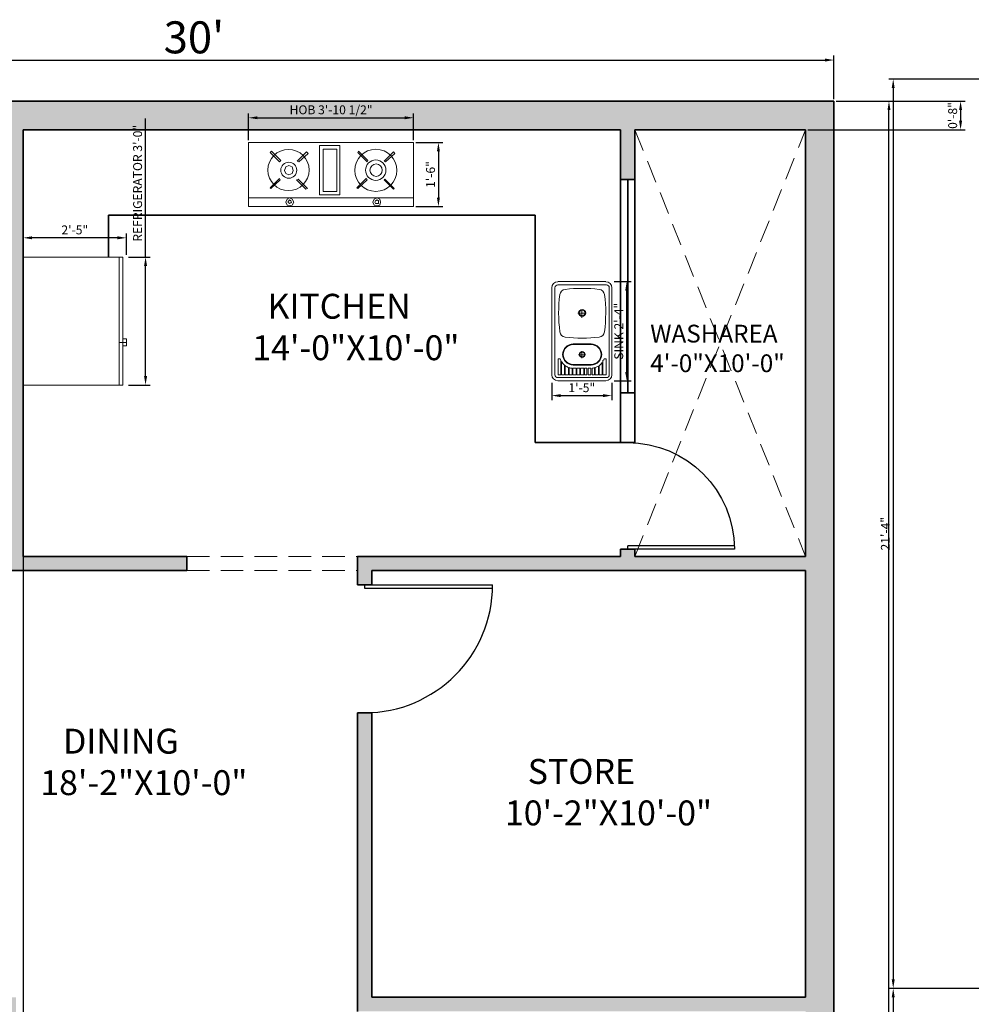
# Model space of a CAD drawing. Units: inches. Extents: x 1566 to 2546, y 1087 to 2705.
# Tile 11 of 27: x 1773 to 2040, y 1524 to 1801. Entities that reach past the tile are written whole.
import ezdxf

# ---------------------------------------------------------------- set-up
doc = ezdxf.new("R2010")
doc.units = ezdxf.units.IN
doc.linetypes.add('DASHED', pattern=[19.05, 12.7, -6.35])
for name, color, linetype, lineweight in [('A-ANNO-DIMS', 2, 'Continuous', 18), ('A-AREA-IDEN', 7, 'Continuous', 18), ('A-DOOR', 4, 'Continuous', 25), ('A-FLOR-FIXT', 9, 'Continuous', 18), ('A-FLOR-OVHD', 8, 'DASHED', 18), ('A-WALL', 7, 'Continuous', 35), ('A-WALL-PATT', 8, 'Continuous', 13)]:
    doc.layers.add(name, color=color, linetype=linetype, lineweight=lineweight)
doc.styles.get("Standard").update_dxf_attribs({"font": 'arial.ttf'})
doc.dimstyles.new('ISO-25', dxfattribs={"dimtxt": 2.5, "dimasz": 2.5, "dimexe": 1.25, "dimexo": 0.625, "dimtad": 1, "dimtxsty": 'Standard', "dimcen": 2.5, "dimadec": 0, "dimazin": 0, "dimtfac": 1, "dimtmove": 0, "dimatfit": 3, "dimfxl": 1, "dimarcsym": 0})

# ---------------------------------------------------------------- blocks, each defined once
blk = doc.blocks.new('d1')
for p, q in [((3297.32, 1596.93), (3297.32, 1632.93)), ((3298.32, 1596.93), (3298.32, 1632.93)), ((3297.32, 1596.93), (3298.32, 1596.93))]:
    blk.add_line(p, q)
at = {"ltscale": 0.3}
blk.add_arc((3297.32, 1596.93), 36, 0, 90, dxfattribs=at)
blk = doc.blocks.new('*D7')
at = {"layer": 'A-ANNO-DIMS', "color": 0, "lineweight": -2, "transparency": 16777216}
for p, q in [((2002.15, 1778.2), (2018.24, 1778.2)), ((2016.99, 1156.7), (2016.99, 1775.7)), ((2002.15, 1154.2), (2018.24, 1154.2))]:
    blk.add_line(p, q, dxfattribs=at)
at = {"layer": 'A-ANNO-DIMS', "color": 0, "transparency": 16777216}
for points in [[(2016.58, 1775.7), (2017.41, 1775.7), (2016.99, 1778.2)], [(2016.58, 1156.7), (2017.41, 1156.7), (2016.99, 1154.2)]]:
    blk.add_solid(points, dxfattribs=at)
at = {"layer": 'Defpoints', "color": 0, "transparency": 16777216}
for p in [(2001.53, 1778.2), (2016.99, 1778.2), (2001.53, 1154.2)]:
    blk.add_point(p, dxfattribs=at)
at = {"layer": 'A-ANNO-DIMS', "color": 0, "transparency": 16777216, "insert": (2011.77, 1466.2), "char_height": 9, "attachment_point": 5, "rotation": 90}
blk.add_mtext("52'", dxfattribs=at)
blk = doc.blocks.new('*D9')
at = {"layer": 'A-ANNO-DIMS', "color": 0, "lineweight": -2, "transparency": 16777216}
for p, q in [((1641.53, 1778.82), (1641.53, 1791.04)), ((1644.03, 1789.79), (1999.03, 1789.79)), ((2001.53, 1778.82), (2001.53, 1791.04))]:
    blk.add_line(p, q, dxfattribs=at)
at = {"layer": 'A-ANNO-DIMS', "color": 0, "transparency": 16777216}
for points in [[(1644.03, 1790.2), (1644.03, 1789.37), (1641.53, 1789.79)], [(1999.03, 1790.2), (1999.03, 1789.37), (2001.53, 1789.79)]]:
    blk.add_solid(points, dxfattribs=at)
at = {"layer": 'Defpoints', "color": 0, "transparency": 16777216}
for p in [(2001.53, 1789.79), (1641.53, 1778.2), (2001.53, 1778.2)]:
    blk.add_point(p, dxfattribs=at)
at = {"layer": 'A-ANNO-DIMS', "color": 0, "transparency": 16777216, "insert": (1821.53, 1795.01), "char_height": 9, "attachment_point": 5}
blk.add_mtext("30'", dxfattribs=at)
blk = doc.blocks.new('d2')
for p, q in [((3364.08, 1632.29), (3364.08, 1602.29)), ((3365.08, 1632.29), (3365.08, 1602.29)), ((3364.08, 1602.29), (3365.08, 1602.29))]:
    blk.add_line(p, q)
at = {"ltscale": 0.3}
blk.add_arc((3364.08, 1602.29), 30, 0, 90, dxfattribs=at)
blk = doc.blocks.new('sink 1')
for points in [[(5.86, 24.22), (-5.86, 24.22)], [(-7.34, 1.48), (-7.34, 22.73)], [(-6.56, 1.48), (-6.56, 22.73)], [(6.01, 23.43), (-5.86, 23.43)], [(6.72, 1.48), (6.72, 22.73)], [(7.34, 1.48), (7.34, 22.73)], [(0, 15.39), (0, 17.42)], [(1.09, 16.48), (-0.94, 16.48)], [(-2.09, 8.99), (2.28, 8.99)], [(-2.09, 8.84), (2.28, 8.84)], [(0, 5.55), (0, 7.26)], [(-5.78, 5.39), (-5.78, 5.39)], [(-5.31, 5.39), (-5.31, 5.39)], [(-5.16, 4.92), (-5.16, 4.92)], [(0.78, 6.33), (-0.78, 6.33)], [(5.16, 4.92), (5.16, 4.92)], [(5.94, 5.39), (5.94, 5.39)], [(-5, 1.48), (-5, 4.69)], [(-5, 1.48), (-4.22, 1.48), (-4.22, 3.83)], [(-4.84, 4.45), (-4.84, 4.45)], [(-4.22, 3.83), (-4.22, 3.83)], [(-4.06, 1.48), (-4.06, 3.69)], [(-4.06, 1.48), (-3.28, 1.48), (-3.28, 3.27)], [(-3.91, 3.52), (-3.91, 3.52)], [(-3.28, 3.2), (-3.28, 3.2)], [(-3.12, 3.2), (-3.12, 3.2)], [(-2.34, 3.05), (-2.34, 3.05)], [(-2.19, 3.05), (-2.19, 3.05)], [(-2.09, 3.99), (2.28, 3.99)], [(-2.09, 3.84), (2.28, 3.84)], [(-1.41, 3.05), (-1.41, 3.05)], [(-1.25, 3.05), (-1.25, 3.05)], [(-0.47, 1.48), (-1.25, 1.48), (-1.25, 3.05), (-0.47, 3.05)], [(-0.62, 3.05), (-0.62, 3.05)], [(-0.47, 1.48), (-0.47, 3.05)], [(-0.31, 3.05), (-0.31, 3.05)], [(0.47, 1.48), (-0.31, 1.48), (-0.31, 3.05), (0.47, 3.05)], [(0.31, 3.05), (0.31, 3.05)], [(0.47, 1.48), (0.47, 3.05)], [(0.62, 3.05), (0.62, 3.05)], [(1.25, 3.05), (1.25, 3.05)], [(1.56, 3.05), (1.56, 3.05)], [(2.19, 3.05), (2.19, 3.05)], [(2.5, 3.05), (2.5, 3.05)], [(3.12, 3.2), (3.12, 3.2)], [(3.28, 1.48), (4.06, 1.48), (4.06, 3.57)], [(3.28, 1.48), (3.28, 3.2)], [(3.44, 3.2), (3.44, 3.2)], [(4.06, 3.52), (4.06, 3.52)], [(4.22, 1.48), (4.22, 3.67)], [(4.37, 3.83), (4.37, 3.83)], [(5, 4.45), (5, 4.45)], [(6.01, 0.78), (-5.86, 0.78)], [(5.86, 0), (-5.86, 0)], [(-5.78, 1.48), (-5.78, 1.48)], [(-5.16, 1.48), (-5.16, 1.48)], [(-4.84, 1.48), (-4.84, 1.48)], [(-4.22, 1.48), (-4.22, 1.48)], [(-3.91, 1.48), (-3.91, 1.48)], [(-3.28, 1.48), (-3.28, 1.48)], [(-3.12, 1.48), (-3.12, 1.48)], [(-2.34, 1.48), (-2.34, 1.48)], [(-2.19, 1.48), (-2.19, 1.48)], [(-1.41, 1.48), (-1.41, 1.48)], [(-1.25, 1.48), (-1.25, 1.48)], [(-0.62, 1.48), (-0.62, 1.48)], [(-0.31, 1.48), (-0.31, 1.48)], [(0.31, 1.48), (0.31, 1.48)], [(0.62, 1.48), (0.62, 1.48)], [(1.25, 1.48), (1.25, 1.48)], [(1.56, 1.48), (1.56, 1.48)], [(2.19, 1.48), (2.19, 1.48)], [(2.5, 1.48), (2.5, 1.48)], [(3.12, 1.48), (3.12, 1.48)], [(3.44, 1.48), (3.44, 1.48)], [(4.06, 1.48), (4.06, 1.48)], [(4.37, 1.48), (4.37, 1.48)], [(5, 1.48), (5, 1.48)], [(5.16, 1.48), (5.16, 1.48)], [(5.94, 1.48), (5.94, 1.48)]]:
    blk.add_lwpolyline(points)
for points in [[(-5.16, 4.92), (-5.16, 1.48), (-5.78, 1.48), (-5.78, 5.39), (-5.31, 5.39, -0.068511), (-5.16, 4.92)], [(5.16, 4.92, 0.248301), (5.47, 5.39), (5.94, 5.39), (5.94, 1.48), (5.16, 1.48), (5.16, 4.92)], [(4.06, 3.57, -0.061679), (3.32, 3.22)], [(4.22, 1.48), (5, 1.48), (5, 4.45, -0.083542), (4.22, 3.67, -0.083542)]]:
    blk.add_lwpolyline(points, format="xyb")
for points in [[(-3.12, 3.22), (-3.12, 1.48), (-2.34, 1.48), (-2.34, 3.05, -0.06228)], [(2.5, 3.05), (2.5, 1.48), (3.12, 1.48), (3.12, 3.2, -0.050256)]]:
    blk.add_lwpolyline(points, format="xyb", close=True)
for points in [[(-2.19, 3.05), (-1.41, 3.05), (-1.41, 1.48), (-2.19, 1.48)], [(0.62, 3.05), (1.25, 3.05), (1.25, 1.48), (0.62, 1.48)], [(2.19, 1.48), (2.19, 3.05), (1.56, 3.05), (1.56, 1.48)]]:
    blk.add_lwpolyline(points, close=True)
for centre, radius in [((0.09, 16.57), 0.859), ((0.09, 16.57), 0.703), ((0.09, 6.41), 0.703), ((0.09, 6.41), 0.547)]:
    blk.add_circle(centre, radius)
for centre, radius, start, end in [((-5.86, 22.73), 1.48, 90, 180), ((5.86, 22.73), 1.48, 360, 90), ((-5.86, 22.73), 0.703, 90, 180), ((-3.87, 20.82), 1.53, 97.3256, 171.1849), ((0.09, -12.65), 35.23, 83.2159, 96.7841), ((4.06, 20.82), 1.53, 8.8151, 82.6744), ((6.01, 22.73), 0.703, 0, 90), ((30.19, 16.56), 35.85, 172.7947, 187.4213), ((-30, 16.56), 35.85, 352.5787, 7.2053), ((-3.89, 12.12), 1.48, 187.4212, 263.2159), ((0.09, 45.63), 35.23, 263.2159, 276.7841), ((4.08, 12.12), 1.48, 276.7841, 352.5788), ((-2.1, 6.41), 2.58, 90, 270), ((-2.1, 6.41), 2.42, 90, 270), ((2.28, 6.41), 2.58, 270, 90), ((2.28, 6.41), 2.42, 270, 90), ((-2.15, 6.48), 3.36, 212.1095, 232.0862), ((-2.1, 6.41), 3.36, 234.156, 249.3275), ((2.14, 6.36), 3.36, 289.8633, 290.5971), ((-5.86, 1.48), 1.48, 180, 270), ((-5.86, 1.48), 0.703, 180, 270), ((5.86, 1.48), 1.48, 270, 0), ((6.01, 1.48), 0.703, 270, 360)]:
    blk.add_arc(centre, radius, start, end)
blk = doc.blocks.new('gas 1')
for points in [[(35.93, -1.87), (35.93, 0), (0, 0), (0, -1.87)], [(8.12, -0.94), (8.44, -1.56), (8.91, -1.87), (9.53, -1.56), (9.84, -0.94), (9.53, -0.31), (8.91, -0.16), (8.44, -0.31)], [(8.59, -0.94), (8.75, -1.25), (8.91, -1.41), (9.22, -1.25), (9.37, -0.94), (9.22, -0.78), (8.91, -0.62), (8.75, -0.78)], [(27.03, -0.94), (27.34, -1.56), (27.97, -1.87), (28.59, -1.56), (28.75, -0.94), (28.59, -0.31), (27.97, -0.16), (27.34, -0.31)], [(27.5, -0.94), (27.65, -1.25), (27.97, -1.41), (28.28, -1.25), (28.28, -0.94), (28.28, -0.62), (27.97, -0.62), (27.65, -0.62)], [(4.84, -3.91), (4.69, -4.06), (6.72, -6.09), (6.87, -5.78)], [(12.81, -3.91), (12.5, -3.75), (10.47, -5.78), (10.78, -5.94)], [(19.84, -13.28), (15.47, -13.28), (15.47, -2.5), (19.84, -2.5)], [(19.22, -12.5), (16.25, -12.5), (16.25, -3.28), (19.22, -3.28)], [(23.75, -3.91), (23.59, -4.06), (25.62, -6.09), (25.78, -5.78)], [(31.71, -3.91), (31.56, -3.75), (29.53, -5.78), (29.68, -5.94)], [(7.81, -7.81), (8.12, -8.59), (8.75, -8.91), (9.53, -8.59), (9.69, -7.81), (9.53, -7.19), (8.75, -6.87), (8.12, -7.19)], [(7.03, -10), (6.72, -9.69), (4.69, -11.72), (5, -12.03)], [(12.97, -11.56), (10.94, -9.69), (10.62, -9.84), (12.65, -11.87)], [(23.75, -11.72), (23.9, -12.03), (25.93, -10), (25.78, -9.69)], [(31.87, -11.56), (29.84, -9.69), (29.53, -9.84), (31.56, -11.87)]]:
    blk.add_lwpolyline(points, close=True)
blk.add_lwpolyline([(35.93, -1.87), (35.93, -13.9), (0, -13.9), (0, -1.87)])
for centre, radius in [((8.7, -7.92), 4.48), ((27.7, -7.86), 4.58), ((8.77, -7.89), 1.74), ((27.69, -7.89), 2.22), ((27.76, -7.89), 1.35)]:
    blk.add_circle(centre, radius)
blk = doc.blocks.new('Refrigerator-2 door - 36 in top')
for p, q in [((0, -26.999999), (36, -26.999999)), ((12, -26.999999), (12, -28.999999)), ((11, -27.999999), (11, -28.999999)), ((11, -28.999999), (13, -28.999999)), ((13, -28.999999), (13, -27.999999))]:
    blk.add_line(p, q)
blk.add_lwpolyline([(0, -27.999999), (0, 0), (36, 0), (36, -27.999999)], close=True)
blk = doc.blocks.new('*D63')
at = {"layer": 'A-ANNO-DIMS', "color": 0, "lineweight": -2, "transparency": 16777216}
for p, q in [((1939.68, 1727.46), (1944.49, 1727.46)), ((1943.24, 1702.09), (1943.24, 1724.96)), ((1939.68, 1699.59), (1944.49, 1699.59))]:
    blk.add_line(p, q, dxfattribs=at)
at = {"layer": 'A-ANNO-DIMS', "color": 0, "transparency": 16777216}
for points in [[(1942.82, 1724.96), (1943.66, 1724.96), (1943.24, 1727.46)], [(1942.82, 1702.09), (1943.66, 1702.09), (1943.24, 1699.59)]]:
    blk.add_solid(points, dxfattribs=at)
at = {"layer": 'Defpoints', "color": 0, "transparency": 16777216}
for p in [(1939.06, 1727.46), (1943.24, 1727.46), (1939.06, 1699.59)]:
    blk.add_point(p, dxfattribs=at)
at = {"layer": 'A-ANNO-DIMS', "color": 0, "transparency": 16777216, "insert": (1941.32, 1713.52), "char_height": 2.5, "attachment_point": 5, "rotation": 90}
blk.add_mtext('SINK 2\'-4"', dxfattribs=at)
blk = doc.blocks.new('*D64')
at = {"layer": 'A-ANNO-DIMS', "color": 0, "lineweight": -2, "transparency": 16777216}
for p, q in [((1922.16, 1698.96), (1922.16, 1694.16)), ((1939.06, 1698.96), (1939.06, 1694.16)), ((1924.66, 1695.41), (1936.56, 1695.41))]:
    blk.add_line(p, q, dxfattribs=at)
at = {"layer": 'A-ANNO-DIMS', "color": 0, "transparency": 16777216}
for points in [[(1924.66, 1695.83), (1924.66, 1694.99), (1922.16, 1695.41)], [(1936.56, 1695.83), (1936.56, 1694.99), (1939.06, 1695.41)]]:
    blk.add_solid(points, dxfattribs=at)
at = {"layer": 'Defpoints', "color": 0, "transparency": 16777216}
for p in [(1922.16, 1699.59), (1939.06, 1699.59), (1939.06, 1695.41)]:
    blk.add_point(p, dxfattribs=at)
at = {"layer": 'A-ANNO-DIMS', "color": 0, "transparency": 16777216, "insert": (1930.61, 1697.31), "char_height": 2.5, "attachment_point": 5}
blk.add_mtext('1\'-5"', dxfattribs=at)
blk = doc.blocks.new('*D65')
at = {"layer": 'A-ANNO-DIMS', "color": 0, "lineweight": -2, "transparency": 16777216}
for p, q in [((1836.88, 1767.21), (1836.88, 1774.8)), ((1839.38, 1773.55), (1880.82, 1773.55)), ((1883.32, 1767.21), (1883.32, 1774.8))]:
    blk.add_line(p, q, dxfattribs=at)
at = {"layer": 'A-ANNO-DIMS', "color": 0, "transparency": 16777216}
for points in [[(1839.38, 1773.97), (1839.38, 1773.14), (1836.88, 1773.55)], [(1880.82, 1773.97), (1880.82, 1773.14), (1883.32, 1773.55)]]:
    blk.add_solid(points, dxfattribs=at)
at = {"layer": 'Defpoints', "color": 0, "transparency": 16777216}
for p in [(1883.32, 1773.55), (1836.88, 1766.59), (1883.32, 1766.59)]:
    blk.add_point(p, dxfattribs=at)
at = {"layer": 'A-ANNO-DIMS', "color": 0, "transparency": 16777216, "insert": (1860.1, 1775.47), "char_height": 2.5, "attachment_point": 5}
blk.add_mtext('HOB 3\'-10 1/2"', dxfattribs=at)
blk = doc.blocks.new('*D66')
at = {"layer": 'A-ANNO-DIMS', "color": 0, "lineweight": -2, "transparency": 16777216}
for p, q in [((1883.95, 1766.59), (1891.54, 1766.59)), ((1890.29, 1764.09), (1890.29, 1751.11)), ((1883.95, 1748.61), (1891.54, 1748.61))]:
    blk.add_line(p, q, dxfattribs=at)
at = {"layer": 'A-ANNO-DIMS', "color": 0, "transparency": 16777216}
for points in [[(1889.87, 1764.09), (1890.71, 1764.09), (1890.29, 1766.59)], [(1889.87, 1751.11), (1890.71, 1751.11), (1890.29, 1748.61)]]:
    blk.add_solid(points, dxfattribs=at)
at = {"layer": 'Defpoints', "color": 0, "transparency": 16777216}
for p in [(1883.32, 1766.59), (1883.32, 1748.61), (1890.29, 1748.61)]:
    blk.add_point(p, dxfattribs=at)
at = {"layer": 'A-ANNO-DIMS', "color": 0, "transparency": 16777216, "insert": (1888.39, 1757.6), "char_height": 2.5, "attachment_point": 5, "rotation": 90}
blk.add_mtext('1\'-6"', dxfattribs=at)
blk = doc.blocks.new('*D67')
at = {"layer": 'A-ANNO-DIMS', "color": 0, "lineweight": -2, "transparency": 16777216}
for p, q in [((1807.93, 1734.39), (1807.93, 1773.37)), ((1803.15, 1734.39), (1809.18, 1734.39)), ((1807.93, 1700.89), (1807.93, 1731.89)), ((1803.15, 1698.39), (1809.18, 1698.39))]:
    blk.add_line(p, q, dxfattribs=at)
at = {"layer": 'A-ANNO-DIMS', "color": 0, "transparency": 16777216}
for points in [[(1807.51, 1731.89), (1808.35, 1731.89), (1807.93, 1734.39)], [(1807.51, 1700.89), (1808.35, 1700.89), (1807.93, 1698.39)]]:
    blk.add_solid(points, dxfattribs=at)
at = {"layer": 'Defpoints', "color": 0, "transparency": 16777216}
for p in [(1802.53, 1734.39), (1807.93, 1734.39), (1802.53, 1698.39)]:
    blk.add_point(p, dxfattribs=at)
at = {"layer": 'A-ANNO-DIMS', "color": 0, "transparency": 16777216, "insert": (1806.01, 1755.13), "char_height": 2.5, "attachment_point": 5, "rotation": 90}
blk.add_mtext('REFRIGERATOR 3\'-0"', dxfattribs=at)
blk = doc.blocks.new('*D68')
at = {"layer": 'A-ANNO-DIMS', "color": 0, "lineweight": -2, "transparency": 16777216}
for p, q in [((1773.53, 1735.01), (1773.53, 1741.04)), ((1800.03, 1739.79), (1776.03, 1739.79)), ((1802.53, 1735.01), (1802.53, 1741.04))]:
    blk.add_line(p, q, dxfattribs=at)
at = {"layer": 'A-ANNO-DIMS', "color": 0, "transparency": 16777216}
for points in [[(1776.03, 1740.21), (1776.03, 1739.37), (1773.53, 1739.79)], [(1800.03, 1740.21), (1800.03, 1739.37), (1802.53, 1739.79)]]:
    blk.add_solid(points, dxfattribs=at)
at = {"layer": 'Defpoints', "color": 0, "transparency": 16777216}
for p in [(1773.53, 1739.79), (1773.53, 1734.39), (1802.53, 1734.39)]:
    blk.add_point(p, dxfattribs=at)
at = {"layer": 'A-ANNO-DIMS', "color": 0, "transparency": 16777216, "insert": (1788.03, 1741.69), "char_height": 2.5, "attachment_point": 5}
blk.add_mtext('2\'-5"', dxfattribs=at)
blk = doc.blocks.new('*D91')
at = {"layer": 'A-ANNO-DIMS', "color": 0, "lineweight": -2, "transparency": 16777216}
for p, q in [((2061.66, 1784.43), (2016.94, 1784.43)), ((2018.19, 1781.93), (2018.19, 1531.18)), ((2061.66, 1528.68), (2016.94, 1528.68))]:
    blk.add_line(p, q, dxfattribs=at)
at = {"layer": 'A-ANNO-DIMS', "color": 0, "transparency": 16777216}
for points in [[(2017.77, 1781.93), (2018.6, 1781.93), (2018.19, 1784.43)], [(2017.77, 1531.18), (2018.6, 1531.18), (2018.19, 1528.68)]]:
    blk.add_solid(points, dxfattribs=at)
at = {"layer": 'Defpoints', "color": 0, "transparency": 16777216}
for p in [(2062.29, 1784.43), (2018.19, 1528.68), (2062.29, 1528.68)]:
    blk.add_point(p, dxfattribs=at)
at = {"layer": 'A-ANNO-DIMS', "color": 0, "transparency": 16777216, "insert": (2016.31, 1656.56), "char_height": 2.5, "attachment_point": 5, "rotation": 90}
blk.add_mtext('21\'-4"', dxfattribs=at)
blk = doc.blocks.new('*D92')
at = {"layer": 'A-ANNO-DIMS', "color": 0, "lineweight": -2, "transparency": 16777216}
for p, q in [((2061.66, 1528.68), (2016.94, 1528.68)), ((2018.19, 1526.18), (2018.19, 1477.15)), ((2061.66, 1474.65), (2016.94, 1474.65))]:
    blk.add_line(p, q, dxfattribs=at)
at = {"layer": 'A-ANNO-DIMS', "color": 0, "transparency": 16777216}
for points in [[(2017.77, 1526.18), (2018.6, 1526.18), (2018.19, 1528.68)], [(2017.77, 1477.15), (2018.6, 1477.15), (2018.19, 1474.65)]]:
    blk.add_solid(points, dxfattribs=at)
at = {"layer": 'Defpoints', "color": 0, "transparency": 16777216}
for p in [(2062.29, 1528.68), (2018.19, 1474.65), (2062.29, 1474.65)]:
    blk.add_point(p, dxfattribs=at)
at = {"layer": 'A-ANNO-DIMS', "color": 0, "transparency": 16777216, "insert": (2016.29, 1501.66), "char_height": 2.5, "attachment_point": 5, "rotation": 90}
blk.add_mtext('4\'-6"', dxfattribs=at)
blk = doc.blocks.new('*D109')
at = {"layer": 'A-ANNO-DIMS', "color": 0, "lineweight": -2, "transparency": 16777216}
for p, q in [((2002.15, 1778.2), (2038.38, 1778.2)), ((2037.13, 1775.7), (2037.13, 1772.7)), ((1994.15, 1770.2), (2038.38, 1770.2))]:
    blk.add_line(p, q, dxfattribs=at)
at = {"layer": 'A-ANNO-DIMS', "color": 0, "transparency": 16777216}
for points in [[(2036.71, 1775.7), (2037.55, 1775.7), (2037.13, 1778.2)], [(2036.71, 1772.7), (2037.55, 1772.7), (2037.13, 1770.2)]]:
    blk.add_solid(points, dxfattribs=at)
at = {"layer": 'Defpoints', "color": 0, "transparency": 16777216}
for p in [(2001.53, 1778.2), (1993.53, 1770.2), (2037.13, 1770.2)]:
    blk.add_point(p, dxfattribs=at)
at = {"layer": 'A-ANNO-DIMS', "color": 0, "transparency": 16777216, "insert": (2035.23, 1774.2), "char_height": 2.5, "attachment_point": 5, "rotation": 90}
blk.add_mtext('0\'-8"', dxfattribs=at)
blk = doc.blocks.new('*D110')
at = {"layer": 'A-ANNO-DIMS', "color": 0, "lineweight": -2, "transparency": 16777216}
for p, q in [((1769.53, 1769.57), (1769.53, 1087.35)), ((1773.53, 1769.57), (1773.53, 1087.35)), ((1767.03, 1088.6), (1764.53, 1088.6)), ((1769.53, 1088.6), (1773.53, 1088.6)), ((1776.03, 1088.6), (1786.43, 1088.6))]:
    blk.add_line(p, q, dxfattribs=at)
at = {"layer": 'A-ANNO-DIMS', "color": 0, "transparency": 16777216}
for points in [[(1767.03, 1089.01), (1767.03, 1088.18), (1769.53, 1088.6)], [(1776.03, 1089.01), (1776.03, 1088.18), (1773.53, 1088.6)]]:
    blk.add_solid(points, dxfattribs=at)
at = {"layer": 'Defpoints', "color": 0, "transparency": 16777216}
for p in [(1769.53, 1770.2), (1773.53, 1770.2), (1773.53, 1088.6)]:
    blk.add_point(p, dxfattribs=at)
at = {"layer": 'A-ANNO-DIMS', "color": 0, "transparency": 16777216, "insert": (1782.48, 1090.5), "char_height": 2.5, "attachment_point": 5}
blk.add_mtext('0\'-4"', dxfattribs=at)

msp = doc.modelspace()

# ---------------------------------------------------------------- hatches: boundary and pattern name
at = {"layer": 'A-WALL-PATT'}
h = msp.add_hatch(color=256, dxfattribs=at)
h.dxf.hatch_style = 1
h.paths.add_polyline_path([(2001.53, 1778.2), (1641.53, 1778.2), (1641.53, 1746.2), (1649.53, 1746.2), (1649.53, 1770.2), (1769.53, 1770.2), (1769.53, 1650.2), (1767.53, 1650.2), (1767.53, 1648.2), (1767.53, 1646.2), (1819.53, 1646.2), (1819.53, 1650.2), (1773.53, 1650.2), (1773.53, 1770.2), (1941.53, 1770.2), (1941.53, 1756.2), (1945.53, 1756.2), (1945.53, 1770.2), (1993.53, 1770.2), (1993.53, 1650.2), (1945.53, 1650.2), (1945.53, 1652.2), (1943.53, 1652.2), (1941.53, 1652.2), (1941.53, 1650.2), (1867.53, 1650.2), (1867.53, 1642.2), (1871.53, 1642.2), (1871.53, 1646.2), (1993.53, 1646.2), (1993.53, 1526.2), (1871.53, 1526.2), (1871.53, 1606.2), (1867.53, 1606.2), (1867.53, 1522.2), (1993.53, 1522.2), (1993.53, 1387.2), (1959.53, 1387.2), (1959.53, 1397.2), (1955.53, 1397.2), (1955.53, 1387.2), (1903.53, 1387.2), (1903.53, 1383.2), (1993.53, 1383.2), (1993.53, 1364.3), (1993.53, 1211.2), (1939.53, 1211.2), (1939.53, 1203.2), (1993.53, 1203.2), (1993.53, 1154.2), (2001.53, 1154.2)])
h.paths.add_polyline_path([(1649.53, 1646.2), (1731.53, 1646.2), (1731.53, 1650.2), (1649.53, 1650.2), (1649.53, 1674.2), (1641.53, 1674.2), (1641.53, 1622.2), (1649.53, 1622.2)], flags=17)
h.paths.add_polyline_path([(1649.53, 1550.2), (1641.53, 1550.2), (1641.53, 1510.2), (1649.53, 1510.2), (1649.53, 1522.2), (1731.53, 1522.2), (1731.53, 1500.2), (1735.53, 1500.2), (1735.53, 1522.2), (1767.53, 1522.2), (1767.53, 1500.2), (1771.53, 1500.2), (1771.53, 1526.2), (1649.53, 1526.2)], flags=17)
h.paths.add_polyline_path([(1649.53, 1464.2), (1735.53, 1464.2), (1735.53, 1470.2), (1731.53, 1470.2), (1731.53, 1468.2), (1649.53, 1468.2), (1649.53, 1480.2), (1641.53, 1480.2), (1641.53, 1419.2), (1649.53, 1419.2)], flags=17)
h.paths.add_polyline_path([(1649.53, 1323.2), (1641.53, 1323.2), (1641.53, 1270.2), (1667.53, 1270.2), (1667.53, 1278.2), (1649.53, 1278.2)], flags=17)
h.paths.add_polyline_path([(1763.53, 1278.2), (1727.53, 1278.2), (1727.53, 1270.2), (1763.53, 1270.2)], flags=17)
h.paths.add_polyline_path([(1823.53, 1383.2), (1827.53, 1383.2), (1827.53, 1385.2), (1827.53, 1387.2), (1819.53, 1387.2), (1819.53, 1324.21), (1819.53, 1278.2), (1811.53, 1278.2), (1811.53, 1274.2), (1811.53, 1270.2), (1819.53, 1270.2), (1819.53, 1203.2), (1877.53, 1203.2), (1877.53, 1211.2), (1823.53, 1211.2)], flags=17)

# ---------------------------------------------------------------- linework, layer by layer
at = {"layer": 'A-FLOR-OVHD', "ltscale": 0.5}
for p, q in [((1945.53, 1770.2), (1993.53, 1650.2)), ((1945.53, 1650.2), (1993.53, 1770.2)), ((1819.53, 1650.2), (1867.53, 1650.2)), ((1819.53, 1646.2), (1867.53, 1646.2))]:
    msp.add_line(p, q, dxfattribs=at)
at = {"layer": 'A-WALL'}
for p, q in [((1641.53, 1778.2), (2001.53, 1778.2)), ((2001.53, 1778.2), (2001.53, 1154.2)), ((1773.53, 1650.2), (1773.53, 1770.2)), ((1773.53, 1770.2), (1941.53, 1770.2)), ((1941.53, 1682.2), (1941.53, 1770.2)), ((1945.53, 1770.2), (1993.53, 1770.2)), ((1945.53, 1682.2), (1945.53, 1770.2)), ((1993.53, 1770.2), (1993.53, 1650.2)), ((1941.53, 1756.2), (1945.53, 1756.2)), ((1943.53, 1756.2), (1943.53, 1696.2)), ((1797.53, 1746.2), (1917.53, 1746.2)), ((1797.53, 1734.39), (1797.53, 1746.2)), ((1917.53, 1682.2), (1917.53, 1746.2)), ((1941.53, 1696.2), (1945.53, 1696.2)), ((1917.53, 1682.2), (1945.53, 1682.2)), ((1941.53, 1650.2), (1941.53, 1652.2)), ((1941.53, 1652.2), (1945.53, 1652.2)), ((1945.53, 1650.2), (1945.53, 1652.2)), ((1773.53, 1650.2), (1819.53, 1650.2)), ((1819.53, 1650.2), (1819.53, 1646.2)), ((1867.53, 1650.2), (1867.53, 1642.2)), ((1867.53, 1650.2), (1941.53, 1650.2)), ((1945.53, 1650.2), (1993.53, 1650.2)), ((1767.53, 1646.2), (1819.53, 1646.2)), ((1871.53, 1646.2), (1871.53, 1642.2)), ((1871.53, 1646.2), (1993.53, 1646.2)), ((1993.53, 1646.2), (1993.53, 1526.2)), ((1867.53, 1642.2), (1871.53, 1642.2)), ((1867.53, 1606.2), (1871.53, 1606.2)), ((1867.53, 1606.2), (1867.53, 1522.2)), ((1871.53, 1606.2), (1871.53, 1526.2)), ((1871.53, 1526.2), (1993.53, 1526.2))]:
    msp.add_line(p, q, dxfattribs=at)

# ---------------------------------------------------------------- block references
at = {"layer": 'A-DOOR', "xscale": -1, "rotation": 270}
msp.add_blockref('d2', (341.24, -1711.88), dxfattribs=at)
at = {"layer": 'A-DOOR', "rotation": 270}
msp.add_blockref('d1', (272.6, 4939.52), dxfattribs=at)
at = {"layer": 'A-FLOR-FIXT', "xscale": -1.292580420916565, "yscale": 1.292580420916565, "zscale": 1.292580420916565, "rotation": 180}
msp.add_blockref('gas 1', (1836.88, 1748.61), dxfattribs=at)
at = {"layer": 'A-FLOR-FIXT', "rotation": 90}
msp.add_blockref('Refrigerator-2 door - 36 in top', (1773.53, 1698.39), dxfattribs=at)
at = {"layer": 'A-FLOR-FIXT', "xscale": 1.150769176553845, "yscale": 1.150769176553845, "zscale": 1.150769176553845}
msp.add_blockref('sink 1', (1930.61, 1699.59), dxfattribs=at)

# ---------------------------------------------------------------- texts
at = {"layer": 'A-AREA-IDEN', "attachment_point": 1}
for s, insert, char_height in [('  KITCHEN\\P14\'-0"X10\'-0"', (1837.94, 1724.04), 7), ('WASHAREA\\P4\'-0"X10\'-0"', (1949.85, 1715.34), 5), ('   DINING\\P18\'-2"X10\'-0"', (1778.3, 1601.71), 7), ('   STORE\\P10\'-2"X10\'-0"', (1908.98, 1593.2), 7)]:
    msp.add_mtext_dynamic_manual_height_columns(s, width=111.7553, gutter_width=12.5, heights=[0], dxfattribs=dict(at, insert=insert, char_height=char_height))

# ---------------------------------------------------------------- dimensions: what is measured, and where the dimension line sits
at = {"layer": 'A-ANNO-DIMS'}
for base, p1, p2, override, picture, middle in [((2001.53, 1789.79), (1641.53, 1778.2), (2001.53, 1778.2), {"dimtxt": 9, "dimdec": 1, "dimlunit": 3, "dimclrd": 0, "dimclre": 0, "dimclrt": 0, "dimtdec": 1}, '*D9', (1821.53, 1795.01)), ((1773.53, 1088.6), (1769.53, 1770.2), (1773.53, 1770.2), {"dimdec": 1, "dimlfac": 1, "dimrnd": 0, "dimzin": 1, "dimdsep": 46, "dimlunit": 4, "dimfrac": 2}, '*D110', (1782.48, 1090.5)), ((1939.06, 1695.41), (1922.16, 1699.59), (1939.06, 1699.59), {"dimdec": 1, "dimrnd": 0, "dimzin": 1, "dimlunit": 4, "dimfrac": 2}, '*D64', (1930.61, 1697.31))]:
    dim = msp.add_linear_dim(base=base, p1=p1, p2=p2, dimstyle='ISO-25', override=override, dxfattribs=at)
    dim.commit()
    dim.dimension.update_dxf_attribs({"geometry": picture, "text_midpoint": middle})
for base, p1, p2, angle, override, picture, middle in [((2018.1868, 1528.6802), (2062.2895, 1784.433), (2062.2895, 1528.6802), 90, {"dimdec": 1, "dimlfac": 1, "dimrnd": 0, "dimzin": 1, "dimdsep": 46, "dimlunit": 4, "dimfrac": 2}, '*D91', (2016.3067, 1656.5566)), ((2037.13, 1770.2), (2001.53, 1778.2), (1993.53, 1770.2), 90, {"dimdec": 1, "dimlfac": 1, "dimrnd": 0, "dimzin": 1, "dimdsep": 46, "dimlunit": 4, "dimfrac": 2}, '*D109', (2035.23, 1774.2)), ((2016.99, 1778.2), (2001.53, 1154.2), (2001.53, 1778.2), 90, {"dimtxt": 9, "dimdec": 1, "dimlunit": 3, "dimclrd": 0, "dimclre": 0, "dimclrt": 0, "dimtdec": 1}, '*D7', (2011.77, 1466.2)), ((1890.29, 1748.61), (1883.32, 1766.59), (1883.32, 1748.61), 270, {"dimdec": 1, "dimrnd": 0, "dimzin": 1, "dimlunit": 4, "dimfrac": 2}, '*D66', (1888.39, 1757.6)), ((1773.53, 1739.79), (1802.53, 1734.39), (1773.53, 1734.39), 180, {"dimdec": 1, "dimrnd": 0, "dimzin": 1, "dimlunit": 4, "dimfrac": 2}, '*D68', (1788.03, 1741.69)), ((2018.19, 1474.65), (2062.29, 1528.68), (2062.29, 1474.65), 90, {"dimdec": 1, "dimlfac": 1, "dimrnd": 0, "dimzin": 1, "dimdsep": 46, "dimlunit": 4, "dimfrac": 2}, '*D92', (2016.29, 1501.66))]:
    dim = msp.add_linear_dim(base=base, p1=p1, p2=p2, angle=angle, dimstyle='ISO-25', override=override, dxfattribs=at)
    dim.commit()
    dim.dimension.update_dxf_attribs({"geometry": picture, "text_midpoint": middle})
dim = msp.add_linear_dim(base=(1883.32, 1773.55), p1=(1836.88, 1766.59), p2=(1883.32, 1766.59), text='HOB <>', dimstyle='ISO-25', override={"dimdec": 1, "dimrnd": 0, "dimzin": 1, "dimlunit": 4, "dimfrac": 2}, dxfattribs=at)
dim.commit()
dim.dimension.update_dxf_attribs({"geometry": '*D65', "text_midpoint": (1860.1, 1775.47)})
for base, p1, p2, text, picture, middle in [((1807.93, 1734.39), (1802.53, 1698.39), (1802.53, 1734.39), 'REFRIGERATOR <>', '*D67', (1806.01, 1755.13)), ((1943.24, 1727.46), (1939.06, 1699.59), (1939.06, 1727.46), 'SINK <>', '*D63', (1941.32, 1713.52))]:
    dim = msp.add_linear_dim(base=base, p1=p1, p2=p2, angle=90, text=text, dimstyle='ISO-25', override={"dimdec": 1, "dimrnd": 0, "dimzin": 1, "dimlunit": 4, "dimfrac": 2}, dxfattribs=at)
    dim.commit()
    dim.dimension.update_dxf_attribs({"geometry": picture, "text_midpoint": middle})

doc.saveas('drawing.dxf')
